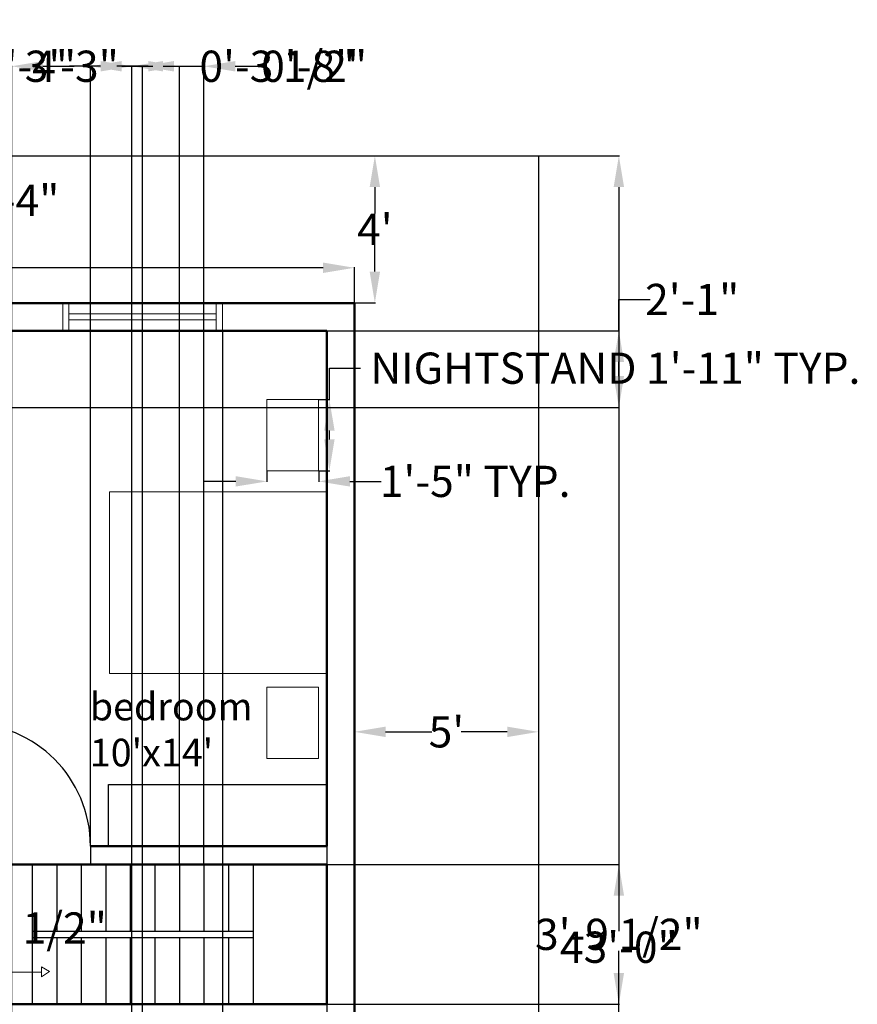
# Model space of a CAD drawing. Units: inches. Extents: x 20 to 3619, y 7 to 1288.
# Tile 4 of 4: x 3346 to 3619, y 967 to 1288. Entities that reach past the tile are written whole.
import ezdxf

# ---------------------------------------------------------------- set-up
doc = ezdxf.new("R2010")
doc.units = ezdxf.units.IN
doc.header["$MEASUREMENT"] = 0
for name, color, linetype, lineweight in [('A-ANNO-DIMS', 2, 'Continuous', 18), ('A-ANNO-SYMB', 7, 'Continuous', 18), ('A-AREA-IDEN', 7, 'Continuous', 25), ('A-DOOR', 3, 'Continuous', 25), ('A-FLOR-CASE', 9, 'Continuous', 25), ('A-FLOR-STRS', 7, 'Continuous', 25), ('A-FURN', 8, 'Continuous', 18), ('A-GLAZ', 4, 'Continuous', 18), ('A-WALL', 7, 'Continuous', 50), ('C-PROP', 8, 'Continuous', 25)]:
    doc.layers.add(name, color=color, linetype=linetype, lineweight=lineweight)
doc.styles.get("Standard").update_dxf_attribs({"font": 'arial.ttf'})
doc.dimstyles.get("Standard").update_dxf_attribs({"dimtxt": 10.18, "dimasz": 10.18, "dimexe": 0.18, "dimexo": 0.0625, "dimgap": 0.09, "dimtad": 0, "dimtih": 1, "dimtoh": 1, "dimdec": 0, "dimzin": 0, "dimdsep": 46, "dimlunit": 3, "dimtxsty": 'Standard', "dimcen": 0.09, "dimadec": 0, "dimazin": 0, "dimtfac": 1, "dimtdec": 0, "dimtofl": 0, "dimtmove": 0, "dimatfit": 3, "dimfxl": 1, "dimtolj": 1, "dimtzin": 0, "dimarcsym": 0})

# ---------------------------------------------------------------- blocks, each defined once
blk = doc.blocks.new('*D3')
at = {"layer": 'A-ANNO-DIMS', "color": 0, "lineweight": -2, "transparency": 16777216}
for p, q in [((3142.72, 1195.76), (3142.72, 1207.38)), ((3152.9, 1207.2), (3289.9, 1207.2)), ((3444.54, 1207.2), (3307.53, 1207.2)), ((3454.72, 1195.76), (3454.72, 1207.38))]:
    blk.add_line(p, q, dxfattribs=at)
at = {"layer": 'A-ANNO-DIMS', "color": 0, "transparency": 16777216}
for points in [[(3152.9, 1208.9), (3152.9, 1205.5), (3142.72, 1207.2)], [(3444.54, 1208.9), (3444.54, 1205.5), (3454.72, 1207.2)]]:
    blk.add_solid(points, dxfattribs=at)
at = {"layer": 'Defpoints', "color": 0, "transparency": 16777216}
for p in [(3454.72, 1207.2), (3142.72, 1195.69), (3454.72, 1195.69)]:
    blk.add_point(p, dxfattribs=at)
at = {"layer": 'A-ANNO-DIMS', "color": 0, "transparency": 16777216, "insert": (3298.72, 1207.2), "char_height": 10.18, "attachment_point": 5}
blk.add_mtext("\\A1;26'", dxfattribs=at)
blk = doc.blocks.new('*D5')
at = {"layer": 'A-ANNO-DIMS', "color": 0, "lineweight": -2, "transparency": 16777216}
for p, q in [((3454.72, 1061.96), (3454.72, 1055.73)), ((3514.72, 1061.96), (3514.72, 1055.73)), ((3464.9, 1055.91), (3479.94, 1055.91)), ((3504.54, 1055.91), (3489.49, 1055.91))]:
    blk.add_line(p, q, dxfattribs=at)
at = {"layer": 'A-ANNO-DIMS', "color": 0, "transparency": 16777216}
for points in [[(3464.9, 1057.61), (3464.9, 1054.21), (3454.72, 1055.91)], [(3504.54, 1057.61), (3504.54, 1054.21), (3514.72, 1055.91)]]:
    blk.add_solid(points, dxfattribs=at)
at = {"layer": 'Defpoints', "color": 0, "transparency": 16777216}
for p in [(3454.72, 1062.03), (3514.72, 1062.03), (3514.72, 1055.91)]:
    blk.add_point(p, dxfattribs=at)
at = {"layer": 'A-ANNO-DIMS', "color": 0, "transparency": 16777216, "insert": (3484.72, 1055.91), "char_height": 10.18, "attachment_point": 5}
blk.add_mtext("\\A1;5'", dxfattribs=at)
blk = doc.blocks.new('*U2')
for p, q in [((0, 0), (0, -6)), ((40, 0), (40, -6))]:
    blk.add_line(p, q)
blk.add_lwpolyline([(0, 0), (0, 40), (1.75, 40), (1.75, 0)], close=True)
blk.add_arc((0, 0), 40, 0, 90)
blk = doc.blocks.new('*D11')
at = {"layer": 'A-ANNO-DIMS', "color": 0, "lineweight": -2, "transparency": 16777216}
for p, q in [((3454.78, 1243.69), (3461.59, 1243.69)), ((3461.41, 1233.51), (3461.41, 1224.9)), ((3461.41, 1205.94), (3461.41, 1214.54)), ((3454.78, 1195.76), (3461.59, 1195.76))]:
    blk.add_line(p, q, dxfattribs=at)
at = {"layer": 'A-ANNO-DIMS', "color": 0, "transparency": 16777216}
for points in [[(3459.71, 1233.51), (3463.1, 1233.51), (3461.41, 1243.69)], [(3459.71, 1205.94), (3463.1, 1205.94), (3461.41, 1195.76)]]:
    blk.add_solid(points, dxfattribs=at)
at = {"layer": 'Defpoints', "color": 0, "transparency": 16777216}
for p in [(3454.72, 1243.69), (3461.41, 1243.69), (3454.72, 1195.76)]:
    blk.add_point(p, dxfattribs=at)
at = {"layer": 'A-ANNO-DIMS', "color": 0, "transparency": 16777216, "insert": (3461.41, 1219.72), "char_height": 10.18, "attachment_point": 5}
blk.add_mtext("\\A1;4'", dxfattribs=at)
blk = doc.blocks.new('WIN-48IN-PLAN')
for p, q in [((0, 0), (0, 9)), ((2, 0), (2, 9)), ((50, 0), (50, 9)), ((52, 0), (52, 9)), ((2, 5.5), (50, 5.5)), ((2, 3.5), (50, 3.5))]:
    blk.add_line(p, q)
blk = doc.blocks.new('BEDSIDE-TABLE')
blk.add_lwpolyline([(0, 23.24), (16.85, 23.24), (16.85, 0), (0, 0)], close=True)
blk = doc.blocks.new('*D26')
at = {"layer": 'A-ANNO-DIMS', "color": 0, "lineweight": -2, "transparency": 16777216}
for p, q in [((3446.58, 1164.29), (3446.58, 1174.47)), ((3446.58, 1174.47), (3456.76, 1174.47)), ((3443.16, 1164.29), (3446.76, 1164.29)), ((3446.58, 1151.23), (3446.58, 1154.11)), ((3443.16, 1141.05), (3446.76, 1141.05))]:
    blk.add_line(p, q, dxfattribs=at)
at = {"layer": 'A-ANNO-DIMS', "color": 0, "transparency": 16777216}
for points in [[(3444.89, 1154.11), (3448.28, 1154.11), (3446.58, 1164.29)], [(3444.89, 1151.23), (3448.28, 1151.23), (3446.58, 1141.05)]]:
    blk.add_solid(points, dxfattribs=at)
at = {"layer": 'Defpoints', "color": 0, "transparency": 16777216}
for p in [(3443.1, 1164.29), (3446.58, 1164.29), (3443.1, 1141.05)]:
    blk.add_point(p, dxfattribs=at)
at = {"layer": 'A-ANNO-DIMS', "color": 0, "transparency": 16777216, "insert": (3539.78, 1174.47), "char_height": 10.18, "attachment_point": 5}
blk.add_mtext('\\A1;NIGHTSTAND 1\'-11" TYP.', dxfattribs=at)
blk = doc.blocks.new('*D27')
at = {"layer": 'A-ANNO-DIMS', "color": 0, "lineweight": -2, "transparency": 16777216}
for p, q in [((3426.24, 1140.99), (3426.24, 1137.38)), ((3443.1, 1140.99), (3443.1, 1137.38)), ((3416.06, 1137.56), (3405.88, 1137.56)), ((3453.28, 1137.56), (3463.46, 1137.56))]:
    blk.add_line(p, q, dxfattribs=at)
at = {"layer": 'A-ANNO-DIMS', "color": 0, "transparency": 16777216}
for points in [[(3416.06, 1139.26), (3416.06, 1135.87), (3426.24, 1137.56)], [(3453.28, 1139.26), (3453.28, 1135.87), (3443.1, 1137.56)]]:
    blk.add_solid(points, dxfattribs=at)
at = {"layer": 'Defpoints', "color": 0, "transparency": 16777216}
for p in [(3426.24, 1141.05), (3443.1, 1141.05), (3443.1, 1137.56)]:
    blk.add_point(p, dxfattribs=at)
at = {"layer": 'A-ANNO-DIMS', "color": 0, "transparency": 16777216, "insert": (3494.09, 1137.56), "char_height": 10.18, "attachment_point": 5}
blk.add_mtext('\\A1;1\'-5" TYP.', dxfattribs=at)
blk = doc.blocks.new('*D28')
at = {"layer": 'A-ANNO-DIMS', "color": 0, "lineweight": -2, "transparency": 16777216}
for p, q in [((3163.42, 1000.64), (3163.42, 991.78)), ((3221.69, 1000.64), (3221.69, 991.78)), ((3173.6, 991.96), (3211.51, 991.96)), ((3221.69, 991.96), (3231.87, 991.96))]:
    blk.add_line(p, q, dxfattribs=at)
at = {"layer": 'A-ANNO-DIMS', "color": 0, "transparency": 16777216}
for points in [[(3173.6, 993.66), (3173.6, 990.26), (3163.42, 991.96)], [(3211.51, 993.66), (3211.51, 990.26), (3221.69, 991.96)]]:
    blk.add_solid(points, dxfattribs=at)
at = {"layer": 'Defpoints', "color": 0, "transparency": 16777216}
for p in [(3163.42, 1000.7), (3221.69, 1000.7), (3221.69, 991.96)]:
    blk.add_point(p, dxfattribs=at)
at = {"layer": 'A-ANNO-DIMS', "color": 0, "transparency": 16777216, "insert": (3303.72, 991.96), "char_height": 10.18, "attachment_point": 5}
blk.add_mtext('\\A1;DINING SET 4\'-10 1/2"', dxfattribs=at)
blk = doc.blocks.new('*D34')
at = {"layer": 'A-ANNO-DIMS', "color": 0, "lineweight": -2, "transparency": 16777216}
for p, q in [((3297.69, 1247.43), (3297.69, 1257.61)), ((3295.33, 1237.25), (3297.87, 1237.25)), ((3295.33, 1221.1), (3297.87, 1221.1)), ((3297.69, 1210.92), (3297.69, 1200.74))]:
    blk.add_line(p, q, dxfattribs=at)
at = {"layer": 'A-ANNO-DIMS', "color": 0, "transparency": 16777216}
for points in [[(3295.99, 1247.43), (3299.38, 1247.43), (3297.69, 1237.25)], [(3295.99, 1210.92), (3299.38, 1210.92), (3297.69, 1221.1)]]:
    blk.add_solid(points, dxfattribs=at)
at = {"layer": 'Defpoints', "color": 0, "transparency": 16777216}
for p in [(3295.27, 1237.25), (3295.27, 1221.1), (3297.69, 1221.1)]:
    blk.add_point(p, dxfattribs=at)
at = {"layer": 'A-ANNO-DIMS', "color": 0, "transparency": 16777216, "insert": (3297.69, 1229.18), "char_height": 10.18, "attachment_point": 5}
blk.add_mtext('\\A1;DISHWASHER 1\'-4"', dxfattribs=at)
blk = doc.blocks.new('*D37')
at = {"layer": 'A-ANNO-DIMS', "color": 0, "lineweight": -2, "transparency": 16777216}
for p, q in [((3514.78, 1243.69), (3541.1, 1243.69)), ((3540.92, 1233.51), (3540.92, 990.98)), ((3540.92, 737.87), (3540.92, 980.4)), ((3514.78, 727.69), (3541.1, 727.69))]:
    blk.add_line(p, q, dxfattribs=at)
at = {"layer": 'A-ANNO-DIMS', "color": 0, "transparency": 16777216}
for points in [[(3539.22, 1233.51), (3542.61, 1233.51), (3540.92, 1243.69)], [(3539.22, 737.87), (3542.61, 737.87), (3540.92, 727.69)]]:
    blk.add_solid(points, dxfattribs=at)
at = {"layer": 'Defpoints', "color": 0, "transparency": 16777216}
for p in [(3514.72, 1243.69), (3540.92, 1243.69), (3514.72, 727.69)]:
    blk.add_point(p, dxfattribs=at)
at = {"layer": 'A-ANNO-DIMS', "color": 0, "transparency": 16777216, "insert": (3540.92, 985.69), "char_height": 10.18, "attachment_point": 5}
blk.add_mtext('\\A1;43\'-0"', dxfattribs=at)
blk = doc.blocks.new('*D40')
at = {"layer": 'A-ANNO-DIMS', "color": 0, "lineweight": -2, "transparency": 16777216}
for p, q in [((3332.89, 1272.89), (3322.71, 1272.89)), ((3343.07, 796.76), (3343.07, 1273.07)), ((3382.22, 796.76), (3382.22, 1273.07)), ((3392.4, 1272.89), (3402.58, 1272.89))]:
    blk.add_line(p, q, dxfattribs=at)
at = {"layer": 'A-ANNO-DIMS', "color": 0, "transparency": 16777216}
for points in [[(3332.89, 1274.59), (3332.89, 1271.2), (3343.07, 1272.89)], [(3392.4, 1274.59), (3392.4, 1271.2), (3382.22, 1272.89)]]:
    blk.add_solid(points, dxfattribs=at)
at = {"layer": 'Defpoints', "color": 0, "transparency": 16777216}
for p in [(3382.22, 1272.89), (3343.07, 796.69), (3382.22, 796.69)]:
    blk.add_point(p, dxfattribs=at)
at = {"layer": 'A-ANNO-DIMS', "color": 0, "transparency": 16777216, "insert": (3362.64, 1272.89), "char_height": 10.18, "attachment_point": 5}
blk.add_mtext('\\A1;3\'-3"', dxfattribs=at)
blk = doc.blocks.new('*D41')
at = {"layer": 'A-ANNO-DIMS', "color": 0, "lineweight": -2, "transparency": 16777216}
for p, q in [((3263.21, 1272.89), (3253.03, 1272.89)), ((3273.39, 796.76), (3273.39, 1273.07)), ((3343.07, 796.76), (3343.07, 1273.07)), ((3353.25, 1272.89), (3363.43, 1272.89))]:
    blk.add_line(p, q, dxfattribs=at)
at = {"layer": 'A-ANNO-DIMS', "color": 0, "transparency": 16777216}
for points in [[(3263.21, 1274.59), (3263.21, 1271.2), (3273.39, 1272.89)], [(3353.25, 1274.59), (3353.25, 1271.2), (3343.07, 1272.89)]]:
    blk.add_solid(points, dxfattribs=at)
at = {"layer": 'Defpoints', "color": 0, "transparency": 16777216}
for p in [(3343.07, 1272.89), (3273.39, 796.69), (3343.07, 796.69)]:
    blk.add_point(p, dxfattribs=at)
at = {"layer": 'A-ANNO-DIMS', "color": 0, "transparency": 16777216, "insert": (3308.23, 1272.89), "char_height": 10.18, "attachment_point": 5}
blk.add_mtext('\\A1;5\'-9 1/2"', dxfattribs=at)
blk = doc.blocks.new('*D42')
at = {"layer": 'A-ANNO-DIMS', "color": 0, "lineweight": -2, "transparency": 16777216}
for p, q in [((3372.04, 1272.89), (3361.86, 1272.89)), ((3382.22, 796.76), (3382.22, 1273.07)), ((3385.72, 796.76), (3385.72, 1273.07)), ((3395.9, 1272.89), (3406.08, 1272.89))]:
    blk.add_line(p, q, dxfattribs=at)
at = {"layer": 'A-ANNO-DIMS', "color": 0, "transparency": 16777216}
for points in [[(3372.04, 1274.59), (3372.04, 1271.2), (3382.22, 1272.89)], [(3395.9, 1274.59), (3395.9, 1271.2), (3385.72, 1272.89)]]:
    blk.add_solid(points, dxfattribs=at)
at = {"layer": 'Defpoints', "color": 0, "transparency": 16777216}
for p in [(3385.72, 1272.89), (3382.22, 796.69), (3385.72, 796.69)]:
    blk.add_point(p, dxfattribs=at)
at = {"layer": 'A-ANNO-DIMS', "color": 0, "transparency": 16777216, "insert": (3431.56, 1272.89), "char_height": 10.18, "attachment_point": 5}
blk.add_mtext('\\A1;0\'-3 1/2"', dxfattribs=at)
blk = doc.blocks.new('*D44')
at = {"layer": 'A-ANNO-DIMS', "color": 0, "lineweight": -2, "transparency": 16777216}
for p, q in [((3540.92, 1186.69), (3540.92, 1196.87)), ((3540.92, 1196.87), (3551.1, 1196.87)), ((3151.78, 1186.69), (3541.1, 1186.69)), ((3540.92, 1171.87), (3540.92, 1176.51)), ((3151.78, 1161.69), (3541.1, 1161.69))]:
    blk.add_line(p, q, dxfattribs=at)
at = {"layer": 'A-ANNO-DIMS', "color": 0, "transparency": 16777216}
for points in [[(3539.22, 1176.51), (3542.61, 1176.51), (3540.92, 1186.69)], [(3539.22, 1171.87), (3542.61, 1171.87), (3540.92, 1161.69)]]:
    blk.add_solid(points, dxfattribs=at)
at = {"layer": 'Defpoints', "color": 0, "transparency": 16777216}
for p in [(3151.72, 1186.69), (3540.92, 1186.69), (3151.72, 1161.69)]:
    blk.add_point(p, dxfattribs=at)
at = {"layer": 'A-ANNO-DIMS', "color": 0, "transparency": 16777216, "insert": (3564.81, 1196.87), "char_height": 10.18, "attachment_point": 5}
blk.add_mtext('\\A1;2\'-1"', dxfattribs=at)
blk = doc.blocks.new('*D45')
at = {"layer": 'A-ANNO-DIMS', "color": 0, "lineweight": -2, "transparency": 16777216}
for p, q in [((3411.72, 1186.63), (3411.72, 701.31)), ((3445.72, 1186.63), (3445.72, 701.31)), ((3421.9, 701.49), (3435.54, 701.49)), ((3445.72, 701.49), (3455.9, 701.49))]:
    blk.add_line(p, q, dxfattribs=at)
at = {"layer": 'A-ANNO-DIMS', "color": 0, "transparency": 16777216}
for points in [[(3421.9, 703.19), (3421.9, 699.8), (3411.72, 701.49)], [(3435.54, 703.19), (3435.54, 699.8), (3445.72, 701.49)]]:
    blk.add_solid(points, dxfattribs=at)
at = {"layer": 'Defpoints', "color": 0, "transparency": 16777216}
for p in [(3411.72, 1186.69), (3445.72, 1186.69), (3445.72, 701.49)]:
    blk.add_point(p, dxfattribs=at)
at = {"layer": 'A-ANNO-DIMS', "color": 0, "transparency": 16777216, "insert": (3473.56, 701.49), "char_height": 10.18, "attachment_point": 5}
blk.add_mtext('\\A1;2\'-10"', dxfattribs=at)
blk = doc.blocks.new('*D48')
at = {"layer": 'A-ANNO-DIMS', "color": 0, "lineweight": -2, "transparency": 16777216}
for p, q in [((3387.54, 1272.89), (3377.36, 1272.89)), ((3397.72, 1012.76), (3397.72, 1273.07)), ((3405.72, 1012.76), (3405.72, 1273.07)), ((3415.9, 1272.89), (3426.08, 1272.89))]:
    blk.add_line(p, q, dxfattribs=at)
at = {"layer": 'A-ANNO-DIMS', "color": 0, "transparency": 16777216}
for points in [[(3387.54, 1274.59), (3387.54, 1271.2), (3397.72, 1272.89)], [(3415.9, 1274.59), (3415.9, 1271.2), (3405.72, 1272.89)]]:
    blk.add_solid(points, dxfattribs=at)
at = {"layer": 'Defpoints', "color": 0, "transparency": 16777216}
for p in [(3405.72, 1272.89), (3397.72, 1012.69), (3405.72, 1012.69)]:
    blk.add_point(p, dxfattribs=at)
at = {"layer": 'A-ANNO-DIMS', "color": 0, "transparency": 16777216, "insert": (3439.7, 1272.89), "char_height": 10.18, "attachment_point": 5}
blk.add_mtext('\\A1;0\'-8"', dxfattribs=at)
blk = doc.blocks.new('*D51')
at = {"layer": 'A-ANNO-DIMS', "color": 0, "lineweight": -2, "transparency": 16777216}
for p, q in [((3445.78, 1012.69), (3541.1, 1012.69)), ((3540.92, 1002.51), (3540.92, 995.25)), ((3540.92, 977.26), (3540.92, 984.53)), ((3445.78, 967.08), (3541.1, 967.08))]:
    blk.add_line(p, q, dxfattribs=at)
at = {"layer": 'A-ANNO-DIMS', "color": 0, "transparency": 16777216}
for points in [[(3539.22, 1002.51), (3542.61, 1002.51), (3540.92, 1012.69)], [(3539.22, 977.26), (3542.61, 977.26), (3540.92, 967.08)]]:
    blk.add_solid(points, dxfattribs=at)
at = {"layer": 'Defpoints', "color": 0, "transparency": 16777216}
for p in [(3445.72, 1012.69), (3540.92, 1012.69), (3445.72, 967.08)]:
    blk.add_point(p, dxfattribs=at)
at = {"layer": 'A-ANNO-DIMS', "color": 0, "transparency": 16777216, "insert": (3540.92, 989.89), "char_height": 10.18, "attachment_point": 5}
blk.add_mtext('\\A1;3\'-9 1/2"', dxfattribs=at)
blk = doc.blocks.new('*D52')
at = {"layer": 'A-ANNO-DIMS', "color": 0, "lineweight": -2, "transparency": 16777216}
for p, q in [((3318.54, 1272.89), (3308.36, 1272.89)), ((3328.72, 1018.76), (3328.72, 1273.07)), ((3368.72, 1018.76), (3368.72, 1273.07)), ((3378.9, 1272.89), (3389.08, 1272.89))]:
    blk.add_line(p, q, dxfattribs=at)
at = {"layer": 'A-ANNO-DIMS', "color": 0, "transparency": 16777216}
for points in [[(3318.54, 1274.59), (3318.54, 1271.2), (3328.72, 1272.89)], [(3378.9, 1274.59), (3378.9, 1271.2), (3368.72, 1272.89)]]:
    blk.add_solid(points, dxfattribs=at)
at = {"layer": 'Defpoints', "color": 0, "transparency": 16777216}
for p in [(3368.72, 1272.89), (3328.72, 1018.69), (3368.72, 1018.69)]:
    blk.add_point(p, dxfattribs=at)
at = {"layer": 'A-ANNO-DIMS', "color": 0, "transparency": 16777216, "insert": (3348.72, 1272.89), "char_height": 10.18, "attachment_point": 5}
blk.add_mtext('\\A1;3\'-4"', dxfattribs=at)

msp = doc.modelspace()

# ---------------------------------------------------------------- linework, layer by layer
at = {"layer": 'A-ANNO-SYMB'}
for p, q in [((3352.72, 977.55), (3352.72, 979.25)), ((3352.72, 979.25), (3352.72, 976.07)), ((3355.34, 977.8), (3352.72, 979.25)), ((3335.85, 977.55), (3352.72, 977.55)), ((3352.72, 976.07), (3355.34, 977.8))]:
    msp.add_line(p, q, dxfattribs=at)
at = {"layer": 'A-FLOR-CASE'}
for p, q in [((3374.57, 1018.69), (3374.57, 1038.73)), ((3374.57, 1038.73), (3445.72, 1038.73))]:
    msp.add_line(p, q, dxfattribs=at)
at = {"layer": 'A-FLOR-STRS'}
for p, q in [((3349.72, 1012.69), (3349.72, 967.08)), ((3357.72, 1012.69), (3357.72, 990.89)), ((3365.72, 1012.69), (3365.72, 990.89)), ((3365.72, 1012.69), (3365.72, 990.89)), ((3373.72, 1012.69), (3373.72, 990.89)), ((3381.72, 1012.69), (3381.72, 990.89)), ((3389.72, 1012.69), (3389.72, 990.89)), ((3397.72, 1012.69), (3397.72, 990.89)), ((3405.72, 1012.69), (3405.72, 990.89)), ((3413.72, 1012.69), (3413.72, 990.89)), ((3421.72, 1012.69), (3421.72, 967.08)), ((3349.72, 990.89), (3421.72, 990.89)), ((3349.72, 988.89), (3421.72, 988.89)), ((3357.72, 988.89), (3357.72, 967.08)), ((3365.72, 988.89), (3365.72, 967.08)), ((3365.72, 988.89), (3365.72, 967.08)), ((3373.72, 988.89), (3373.72, 967.08)), ((3381.72, 988.89), (3381.72, 967.08)), ((3389.72, 988.89), (3389.72, 967.08)), ((3397.72, 988.89), (3397.72, 967.08)), ((3405.72, 988.89), (3405.72, 967.08)), ((3413.72, 988.89), (3413.72, 967.08))]:
    msp.add_line(p, q, dxfattribs=at)
at = {"layer": 'A-FURN'}
msp.add_lwpolyline([(3445.72, 1134.16), (3374.96, 1134.16), (3374.96, 1074.97), (3445.72, 1074.97)], close=True, dxfattribs=at)
at = {"layer": 'A-WALL'}
for p, q in [((3218.06, 1195.69), (3454.72, 1195.69)), ((3454.72, 1195.69), (3454.72, 958.08)), ((3325.72, 1186.69), (3445.72, 1186.69)), ((3445.72, 1186.69), (3445.72, 1018.69)), ((3368.72, 1018.69), (3445.72, 1018.69)), ((3328.72, 1012.69), (3445.72, 1012.69)), ((3445.72, 1012.69), (3445.72, 967.08)), ((3445.72, 967.08), (3319.72, 967.08))]:
    msp.add_line(p, q, dxfattribs=at)
at = {"layer": 'C-PROP'}
for p, q in [((3142.72, 1243.69), (3514.72, 1243.69)), ((3514.72, 1243.69), (3514.72, 727.69))]:
    msp.add_line(p, q, dxfattribs=at)

# ---------------------------------------------------------------- block references
at = {"layer": 'A-DOOR'}
msp.add_blockref('*U2', (3328.72, 1018.69), dxfattribs=at)
at = {"layer": 'A-FURN'}
for p in [(3426.24, 1141.05), (3426.24, 1047.25)]:
    msp.add_blockref('BEDSIDE-TABLE', p, dxfattribs=at)
at = {"layer": 'A-GLAZ'}
msp.add_blockref('WIN-48IN-PLAN', (3359.72, 1186.69), dxfattribs=at)

# ---------------------------------------------------------------- texts
at = {"layer": 'A-AREA-IDEN', "insert": (3368.52, 1068.65), "char_height": 9, "attachment_point": 1}
msp.add_mtext_dynamic_manual_height_columns("bedroom\\P10'x14' ", width=17.3739, gutter_width=1, heights=[0], dxfattribs=at)

# ---------------------------------------------------------------- dimensions: what is measured, and where the dimension line sits
at = {"layer": 'A-ANNO-DIMS'}
for base, p1, p2, override, picture, middle in [((3343.07, 1272.89), (3273.39, 796.69), (3343.07, 796.69), {"dimdec": 1, "dimlfac": 1, "dimrnd": 0, "dimzin": 1, "dimdsep": 46, "dimlunit": 4, "dimfrac": 2}, '*D41', (3308.23, 1272.89)), ((3385.72, 1272.89), (3382.22, 796.69), (3385.72, 796.69), {"dimdec": 1, "dimlfac": 1, "dimrnd": 0, "dimzin": 1, "dimdsep": 46, "dimlunit": 4, "dimfrac": 2}, '*D42', (3431.56, 1272.89)), ((3368.72, 1272.89), (3328.72, 1018.69), (3368.72, 1018.69), {"dimdec": 1, "dimlfac": 1, "dimrnd": 0, "dimzin": 1, "dimdsep": 46, "dimlunit": 4, "dimfrac": 2}, '*D52', (3348.72, 1272.89)), ((3382.2188, 1272.8933), (3343.0711, 796.6933), (3382.2188, 796.6933), {"dimdec": 1, "dimlfac": 1, "dimrnd": 0, "dimzin": 1, "dimdsep": 46, "dimlunit": 4, "dimfrac": 2}, '*D40', (3362.6449, 1272.8933)), ((3405.72, 1272.89), (3397.72, 1012.69), (3405.72, 1012.69), {"dimdec": 1, "dimlfac": 1, "dimrnd": 0, "dimzin": 1, "dimdsep": 46, "dimlunit": 4, "dimfrac": 2}, '*D48', (3439.7, 1272.89)), ((3454.72, 1207.2), (3142.72, 1195.69), (3454.72, 1195.69), {"dimclrd": 0, "dimclre": 0, "dimclrt": 0}, '*D3', (3298.72, 1207.2)), ((3445.72, 701.49), (3411.72, 1186.69), (3445.72, 1186.69), {"dimdec": 1, "dimlfac": 1, "dimrnd": 0, "dimzin": 1, "dimdsep": 46, "dimlunit": 4, "dimfrac": 2}, '*D45', (3473.56, 701.49)), ((3514.72, 1055.91), (3454.72, 1062.03), (3514.72, 1062.03), {"dimclrd": 0, "dimclre": 0, "dimclrt": 0}, '*D5', (3484.72, 1055.91))]:
    dim = msp.add_linear_dim(base=base, p1=p1, p2=p2, dimstyle='Standard', override=override, dxfattribs=at)
    dim.commit()
    dim.dimension.update_dxf_attribs({"geometry": picture, "text_midpoint": middle})
for base, p1, p2, angle, text, picture, middle in [((3297.6875, 1221.1016), (3295.2652, 1237.2503), (3295.2652, 1221.1016), 270, 'DISHWASHER <>', '*D34', (3297.6875, 1229.1759)), ((3446.58, 1164.29), (3443.1, 1141.05), (3443.1, 1164.29), 90, 'NIGHTSTAND <> TYP.', '*D26', (3539.78, 1174.47))]:
    dim = msp.add_linear_dim(base=base, p1=p1, p2=p2, angle=angle, text=text, dimstyle='Standard', override={"dimdec": 1, "dimlfac": 1, "dimrnd": 0, "dimzin": 1, "dimdsep": 46, "dimlunit": 4, "dimfrac": 2}, dxfattribs=at)
    dim.commit()
    dim.dimension.update_dxf_attribs({"geometry": picture, "text_midpoint": middle})
for base, p1, p2, override, picture, middle in [((3461.41, 1243.69), (3454.72, 1195.76), (3454.72, 1243.69), {"dimclrd": 0, "dimclre": 0, "dimclrt": 0}, '*D11', (3461.41, 1219.72)), ((3540.92, 1243.69), (3514.72, 727.69), (3514.72, 1243.69), {"dimdec": 1, "dimlfac": 1, "dimrnd": 0, "dimzin": 1, "dimdsep": 46, "dimlunit": 4, "dimfrac": 2}, '*D37', (3540.92, 985.69)), ((3540.92, 1186.69), (3151.72, 1161.69), (3151.72, 1186.69), {"dimdec": 1, "dimlfac": 1, "dimrnd": 0, "dimzin": 1, "dimdsep": 46, "dimlunit": 4, "dimfrac": 2}, '*D44', (3564.81, 1196.87)), ((3540.92, 1012.69), (3445.72, 967.08), (3445.72, 1012.69), {"dimdec": 1, "dimlfac": 1, "dimrnd": 0, "dimzin": 1, "dimdsep": 46, "dimlunit": 4, "dimfrac": 2}, '*D51', (3540.92, 989.89))]:
    dim = msp.add_linear_dim(base=base, p1=p1, p2=p2, angle=90, dimstyle='Standard', override=override, dxfattribs=at)
    dim.commit()
    dim.dimension.update_dxf_attribs({"geometry": picture, "text_midpoint": middle})
for base, p1, p2, text, picture, middle in [((3443.1, 1137.56), (3426.24, 1141.05), (3443.1, 1141.05), '<> TYP.', '*D27', (3494.09, 1137.56)), ((3221.69, 991.96), (3163.42, 1000.7), (3221.69, 1000.7), 'DINING SET <>', '*D28', (3303.72, 991.96))]:
    dim = msp.add_linear_dim(base=base, p1=p1, p2=p2, text=text, dimstyle='Standard', override={"dimdec": 1, "dimlfac": 1, "dimrnd": 0, "dimzin": 1, "dimdsep": 46, "dimlunit": 4, "dimfrac": 2}, dxfattribs=at)
    dim.commit()
    dim.dimension.update_dxf_attribs({"geometry": picture, "text_midpoint": middle})

doc.saveas('drawing.dxf')
